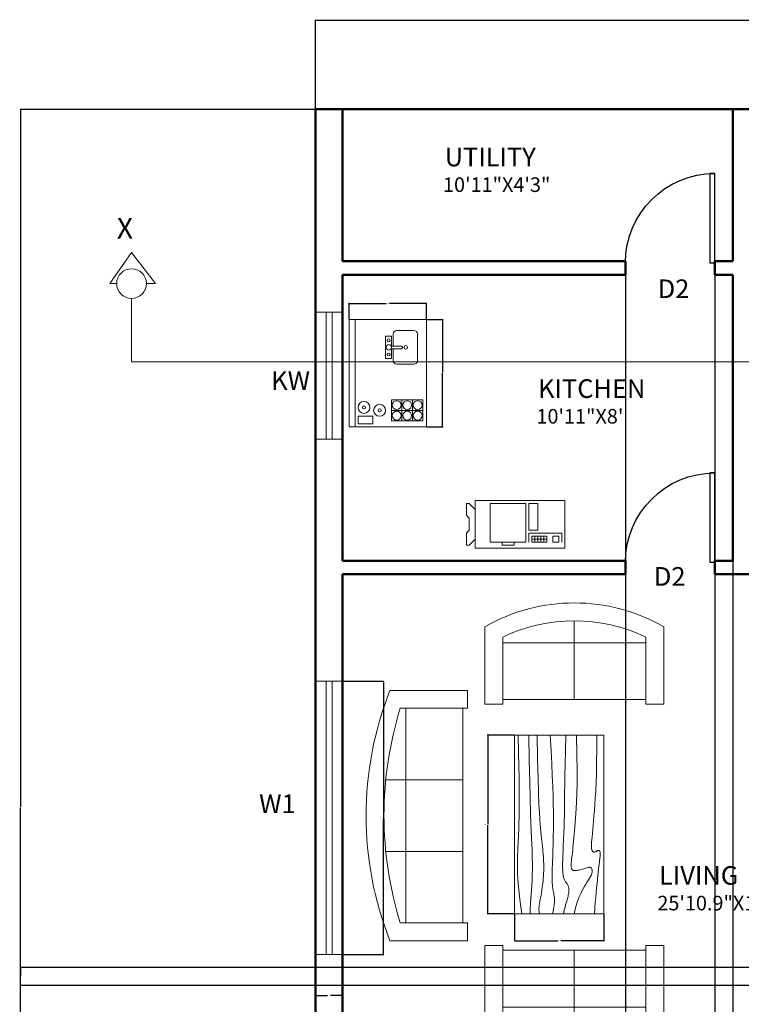
# Model space of a CAD drawing. Units: inches. Extents: x 7359 to 7979, y 33027 to 34263.
# Tile 31 of 32: x 7359 to 7601, y 33933 to 34263. Entities that reach past the tile are written whole.
import ezdxf

# ---------------------------------------------------------------- set-up
doc = ezdxf.new("R2010")
doc.units = ezdxf.units.IN
for name, color, linetype, lineweight in [('A-ANNO-DIMS', 2, 'Continuous', 18), ('A-ANNO-SYMB', 7, 'Continuous', 18), ('A-ANNO-TEXT', 3, 'Continuous', 18), ('A-AREA-IDEN', 7, 'Continuous', 18), ('A-DOOR', 3, 'Continuous', 25), ('A-EQPM', 8, 'Continuous', 18), ('A-FLOR-FIXT', 9, 'Continuous', 18), ('A-FURN', 8, 'Continuous', 18), ('A-GLAZ', 4, 'Continuous', 18), ('A-WALL', 7, 'Continuous', 50)]:
    doc.layers.add(name, color=color, linetype=linetype, lineweight=lineweight)
doc.styles.get("Standard").update_dxf_attribs({"font": 'arial.ttf'})
doc.dimstyles.get("Standard").update_dxf_attribs({"dimtxt": 0.18, "dimasz": 0.18, "dimexe": 0.18, "dimexo": 0.0625, "dimgap": 0.09, "dimtad": 0, "dimtih": 1, "dimtoh": 1, "dimdec": 4, "dimzin": 0, "dimdsep": 46, "dimtxsty": 'Standard', "dimcen": 0.09, "dimadec": 0, "dimazin": 0, "dimtfac": 1, "dimtdec": 4, "dimtofl": 0, "dimtmove": 0, "dimatfit": 3, "dimfxl": 1, "dimtolj": 1, "dimtzin": 0, "dimarcsym": 0})

# ---------------------------------------------------------------- blocks, each defined once
blk = doc.blocks.new('*U2')
for p, q in [((0, 0), (0, -100)), ((750, 0), (750, -100))]:
    blk.add_line(p, q)
blk.add_lwpolyline([(0, 0), (0, 750), (43.75, 750), (43.75, 0)], close=True)
blk.add_arc((0, 0), 750, 0, 90)
blk = doc.blocks.new('Table - Rectangular Woodgrain 60 x 30 in.')
for p, q in [((0, 0), (0, -30)), ((60, 0), (0, 0)), ((60, -30), (60, 0)), ((0, -30), (60, -30))]:
    blk.add_line(p, q)
for points in [[(0, -2.4), (4.8155, -2.418), (9.0302, -2.4688), (12.709, -2.5477), (15.9167, -2.65), (18.7181, -2.7711), (21.1781, -2.9063), (23.3616, -3.0508), (25.3333, -3.2), (27.1477, -3.3495), (28.8172, -3.4958), (30.3437, -3.636), (31.7291, -3.7667), (32.9756, -3.8849), (34.0849, -3.9875), (35.059, -4.0714), (35.9, -4.1334), (36.6114, -4.1711), (37.2041, -4.1854), (37.6906, -4.1779), (38.0833, -4.15), (38.3948, -4.1034), (38.6375, -4.0396), (38.8239, -3.9602), (38.9666, -3.8667), (39.0764, -3.7608), (39.1573, -3.6448), (39.2116, -3.521), (39.2416, -3.3917), (39.2498, -3.2593), (39.2385, -3.1261), (39.21, -2.9944), (39.1666, -2.8667), (39.111, -2.7447), (39.0468, -2.6281), (38.978, -2.5163), (38.9083, -2.4083), (38.8418, -2.3035), (38.7823, -2.201), (38.7337, -2.1001), (38.7, -2), (38.6844, -1.9003), (38.6875, -1.8021), (38.7094, -1.707), (38.75, -1.6167), (38.8094, -1.5326), (38.8875, -1.4563), (38.9844, -1.3893), (39.1, -1.3333), (39.2351, -1.2896), (39.3937, -1.2583), (39.5804, -1.2396), (39.8, -1.2333), (40.057, -1.2396), (40.3562, -1.2583), (40.7023, -1.2896), (41.1, -1.3333), (41.5547, -1.3895), (42.0755, -1.4573), (42.6721, -1.5361), (43.3542, -1.625), (44.1316, -1.7233), (45.014, -1.8302), (46.0114, -1.9449), (47.1333, -2.0667), (48.3862, -2.1947), (49.7625, -2.3281), (51.2513, -2.4663), (52.8416, -2.6083), (54.5226, -2.7535), (56.2833, -2.9011), (58.1127, -3.0501), (60, -3.2)], [(0, -9.2), (6.5759, -9.0858), (11.9385, -9.0365), (16.2527, -9.0418), (19.6833, -9.0917), (22.3952, -9.1759), (24.5531, -9.2844), (26.322, -9.4069), (27.8666, -9.5333), (29.3241, -9.6553), (30.7203, -9.7719), (32.0532, -9.8837), (33.3208, -9.9917), (34.5213, -10.0965), (35.6526, -10.199), (36.7128, -10.2999), (37.7, -10.4), (38.6129, -10.4996), (39.4531, -10.5969), (40.223, -10.6895), (40.925, -10.775), (41.5613, -10.8512), (42.1344, -10.9156), (42.6465, -10.966), (43.1, -11), (43.4976, -11.0158), (43.8437, -11.0136), (44.143, -10.9942), (44.4, -10.9583), (44.6195, -10.9069), (44.8062, -10.8406), (44.9648, -10.7603), (45.1, -10.6667), (45.2155, -10.5598), (45.3114, -10.4365), (45.3871, -10.2929), (45.4416, -10.125), (45.4743, -9.929), (45.4844, -9.7011), (45.4709, -9.4371), (45.4333, -9.1333), (45.3716, -8.7883), (45.2896, -8.4104), (45.1919, -8.0107), (45.0833, -7.6), (44.9685, -7.1893), (44.8521, -6.7896), (44.7388, -6.4117), (44.6333, -6.0667), (44.54, -5.7628), (44.4614, -5.4979), (44.4001, -5.2675), (44.3583, -5.0667), (44.3384, -4.8909), (44.3427, -4.7354), (44.3736, -4.5956), (44.4333, -4.4667), (44.5236, -4.3453), (44.6427, -4.2333), (44.7884, -4.1339), (44.9583, -4.05), (45.1501, -3.9849), (45.3614, -3.9417), (45.59, -3.9234), (45.8333, -3.9333), (46.0915, -3.9749), (46.3734, -4.0531), (46.6906, -4.1736), (47.0542, -4.3417), (47.4756, -4.5629), (47.9661, -4.8427), (48.5372, -5.1866), (49.2, -5.6), (49.9676, -6.0844), (50.8594, -6.625), (51.8965, -7.2031), (53.1, -7.8), (54.491, -8.3969), (56.0906, -8.975), (57.9199, -9.5156), (60, -10)], [(0, -12.8), (5.1847, -12.9322), (9.6213, -13.0323), (13.3963, -13.1059), (16.5958, -13.1583), (19.3063, -13.1952), (21.614, -13.2219), (23.6054, -13.2439), (25.3666, -13.2667), (26.9728, -13.2947), (28.4531, -13.3281), (29.8256, -13.3663), (31.1083, -13.4083), (32.3191, -13.4535), (33.476, -13.501), (34.597, -13.5501), (35.7, -13.6), (36.7984, -13.6497), (37.8875, -13.6979), (38.9578, -13.743), (40, -13.7833), (41.0047, -13.8174), (41.9625, -13.8438), (42.864, -13.8607), (43.7, -13.8667), (44.4631, -13.8604), (45.1552, -13.8417), (45.7801, -13.8104), (46.3416, -13.7667), (46.8439, -13.7104), (47.2906, -13.6417), (47.6858, -13.5604), (48.0333, -13.4667), (48.3375, -13.3608), (48.6042, -13.2448), (48.8396, -13.121), (49.05, -12.9917), (49.2417, -12.8593), (49.4208, -12.7261), (49.5937, -12.5944), (49.7667, -12.4667), (49.9452, -12.3451), (50.1323, -12.2313), (50.3303, -12.1268), (50.5416, -12.0333), (50.7686, -11.9524), (51.0135, -11.8854), (51.2788, -11.8341), (51.5666, -11.8), (51.8785, -11.7843), (52.2116, -11.7865), (52.562, -11.8059), (52.926, -11.8417), (53.2998, -11.8931), (53.6795, -11.9594), (54.0614, -12.0397), (54.4416, -12.1333), (54.8223, -12.2401), (55.2293, -12.3625), (55.6942, -12.5037), (56.2489, -12.6667), (56.9251, -12.8547), (57.7545, -13.0708), (58.7689, -13.3182), (60, -13.6)], [(0, -18), (5.124, -17.7273), (9.6609, -17.5057), (13.6705, -17.3303), (17.2125, -17.1958), (20.3467, -17.0973), (23.1328, -17.0297), (25.6307, -16.9878), (27.9, -16.9667), (29.9928, -16.9617), (31.9302, -16.9703), (33.7254, -16.9907), (35.3917, -17.0208), (36.9423, -17.0588), (38.3906, -17.1026), (39.7499, -17.1503), (41.0333, -17.2), (42.2519, -17.2496), (43.4073, -17.2969), (44.4986, -17.3395), (45.525, -17.375), (46.4858, -17.4012), (47.3802, -17.4156), (48.2074, -17.416), (48.9667, -17.4), (49.6583, -17.3662), (50.2872, -17.3167), (50.8595, -17.2547), (51.3812, -17.1833), (51.8584, -17.1057), (52.2971, -17.025), (52.7034, -16.9443), (53.0833, -16.8667), (53.443, -16.7951), (53.789, -16.7313), (54.128, -16.6768), (54.4666, -16.6334), (54.8115, -16.6024), (55.1693, -16.5854), (55.5465, -16.5841), (55.95, -16.6), (56.3828, -16.6337), (56.8346, -16.6823), (57.2915, -16.7418), (57.7396, -16.8084), (58.165, -16.878), (58.5539, -16.9469), (58.8924, -17.0111), (59.1666, -17.0667), (59.3679, -17.1107), (59.5078, -17.1438), (59.6032, -17.1675), (59.6708, -17.1833), (59.7275, -17.193), (59.7901, -17.1979), (59.8753, -17.1998), (60, -17.2)], [(0, -22.4), (8.0098, -22.2501), (14.4094, -22.1011), (19.4168, -21.9535), (23.25, -21.8083), (26.1269, -21.6663), (28.2656, -21.5281), (29.884, -21.3947), (31.2, -21.2667), (32.3967, -21.1448), (33.5172, -21.0292), (34.5697, -20.9198), (35.5625, -20.8167), (36.5037, -20.7198), (37.4015, -20.6292), (38.2642, -20.5448), (39.1, -20.4667), (39.9164, -20.3951), (40.7187, -20.3313), (41.5117, -20.2768), (42.3, -20.2333), (43.0883, -20.2024), (43.8812, -20.1854), (44.6836, -20.1841), (45.5, -20.2), (46.3328, -20.234), (47.1747, -20.2844), (48.0163, -20.3488), (48.8479, -20.425), (49.66, -20.5106), (50.4429, -20.6031), (51.1872, -20.7004), (51.8833, -20.8), (52.5246, -20.8999), (53.1166, -20.9995), (53.6681, -21.0983), (54.1875, -21.1958), (54.6834, -21.2919), (55.1646, -21.3859), (55.6394, -21.4777), (56.1167, -21.5667), (56.6028, -21.6515), (57.0961, -21.7266), (57.5929, -21.7852), (58.0896, -21.8208), (58.5823, -21.8268), (59.0674, -21.7964), (59.5412, -21.723), (60, -21.6)], [(0, -25.2), (8.6355, -25.0504), (15.7026, -24.9031), (21.4049, -24.7606), (25.9458, -24.625), (29.529, -24.4988), (32.3578, -24.3844), (34.6359, -24.284), (36.5667, -24.2), (38.3213, -24.1341), (39.9417, -24.0854), (41.437, -24.0523), (42.8167, -24.0333), (44.0901, -24.0268), (45.2667, -24.0313), (46.3557, -24.0451), (47.3667, -24.0667), (48.309, -24.0947), (49.1928, -24.1287), (50.0284, -24.168), (50.826, -24.2125), (51.5959, -24.2617), (52.3483, -24.3151), (53.0935, -24.3725), (53.8417, -24.4334), (54.6009, -24.497), (55.3699, -24.561), (56.1454, -24.6226), (56.9239, -24.6792), (57.7021, -24.7279), (58.4764, -24.7662), (59.2435, -24.7911), (60, -24.8)], [(0, -28.8), (5.6867, -28.6681), (10.45, -28.5698), (14.407, -28.5012), (17.675, -28.4584), (20.3711, -28.4374), (22.6125, -28.4344), (24.5164, -28.4455), (26.2, -28.4667), (27.762, -28.4947), (29.2276, -28.5281), (30.6033, -28.5663), (31.8958, -28.6084), (33.1118, -28.6535), (34.2578, -28.7011), (35.3405, -28.7501), (36.3666, -28.8), (37.3443, -28.8497), (38.288, -28.8974), (39.2137, -28.9412), (40.1375, -28.9792), (41.0753, -29.0093), (42.0432, -29.0297), (43.0572, -29.0384), (44.1333, -29.0333), (45.2936, -29.0114), (46.5843, -28.9641), (48.0579, -28.8816), (49.7666, -28.7542), (51.7629, -28.5721), (54.0989, -28.3255), (56.8272, -28.0048), (60, -27.6)]]:
    blk.add_lwpolyline(points)
blk = doc.blocks.new('Sofa - Roundback 7 ft.')
for p, q in [((-12.00002, -32.4421), (-12.00003, -6.5971)), ((11.99997, -32.4421), (11.99998, -6.5971)), ((-36.000027, -34), (-36.000027, -11.4696)), ((35.99998, -34), (35.99998, -11.4696)), ((-35.999844, -13.3819), (35.9998, -13.3819)), ((-36.000027, -32.4421), (35.99998, -32.4421))]:
    blk.add_line(p, q)
for points in [[(-36.000027, -34), (-42.000027, -34), (-42.000027, -8)], [(41.99998, -8), (41.99998, -34), (35.99998, -34)]]:
    blk.add_lwpolyline(points)
for centre, radius, start, end in [((0, -114.25), 114.25, 68.43141, 111.5686), ((-0.00001, -127.1968), 121.1968, 72.72033, 107.2797)]:
    blk.add_arc(centre, radius, start, end)
blk = doc.blocks.new('Sofa - Roundback Loveseat 5 ft.')
for p, q in [((0, -32.44198), (0, -5.99998)), ((-24, -33.99998), (-24, -11.46958)), ((24.00004, -33.99998), (24.00004, -11.46958)), ((-23.9998, -13.38178), (23.99986, -13.38178)), ((-24, -32.44198), (24.00004, -32.44198))]:
    blk.add_line(p, q)
for points in [[(-24, -33.99998), (-30, -33.99998), (-30, -7.99998)], [(30.00004, -7.99998), (30.00004, -33.99998), (24.00004, -33.99998)]]:
    blk.add_lwpolyline(points)
for centre, radius, start, end in [((0, -60.24998), 60.24998, 60.13715, 119.8628), ((0, -61.38438), 55.38444, 64.32083, 115.6792)]:
    blk.add_arc(centre, radius, start, end)
blk = doc.blocks.new('Wet Bar')
for p, q in [((0, 0), (36, 0)), ((0, -26), (0, 0)), ((36, 0), (36, -26)), ((0, -2), (36, -2)), ((3.5, -3), (1, -3)), ((1, -3), (1, -8)), ((3.5, -8), (3.5, -3)), ((1, -8), (3.5, -8)), ((2, -14.25), (9, -14.25)), ((2, -24.75), (2, -14.25)), ((5.5, -14.25), (5.5, -24.75)), ((9, -14.25), (9, -24.75)), ((26.2, -17.55), (26.2, -14.1284)), ((27.1001, -17.55), (27.1001, -14.1284)), ((2, -17.75), (9, -17.75)), ((9, -21.25), (2, -21.25)), ((36, -26), (0, -26)), ((9, -24.75), (2, -24.75))]:
    blk.add_line(p, q)
for points in [[(26.2, -14.25), (22.95, -14.25), (22.95, -12.2), (26.75, -12.2)], [(26.7487, -12.2), (30.3501, -12.2), (30.3501, -14.25), (27.1001, -14.25)], [(20.95, -21.75), (20.95, -16.05)], [(22.15, -14.85), (26.2, -14.85)], [(27.1001, -14.85), (31.15, -14.85)], [(32.3501, -16.05), (32.3501, -21.75)], [(31.15, -22.95), (22.15, -22.95)]]:
    blk.add_lwpolyline(points)
for centre, radius in [((6.5, -5), 2), ((6.5, -5), 0.5), ((5.5, -10.25), 2), ((5.5, -10.25), 0.5), ((24.25, -13.25), 0.5), ((26.65, -13.35), 0.9), ((29, -13.25), 0.5), ((3.75, -16), 1.5), ((7.25, -16), 1.5), ((3.75, -19.5), 1.5), ((7.25, -19.5), 1.5), ((26.65, -19.05), 0.6), ((3.75, -23), 1.5), ((7.25, -23), 1.5)]:
    blk.add_circle(centre, radius)
for centre, radius, start, end in [((22.2251, -16.125), 1.2772, 93.36646, 176.6335), ((31.075, -16.125), 1.2772, 3.366461, 86.63354), ((26.65, -17.55), 0.45, 180, 0), ((22.2251, -21.675), 1.2772, 183.3665, 266.6335), ((31.075, -21.675), 1.2772, 273.3665, 356.6335)]:
    blk.add_arc(centre, radius, start, end)
blk = doc.blocks.new('Copy Machine')
for p, q in [((0, 0), (0, -16)), ((30, 0), (0, 0)), ((30, -16), (30, 0)), ((-3, -1), (-3, -5)), ((-2, -1), (-3, -1)), ((0, -3), (-2, -1)), ((5, -1), (5, -14)), ((17, -1), (5, -1)), ((17, -14), (17, -1)), ((18, -1), (18, -10)), ((21, -1), (18, -1)), ((21, -10), (21, -1)), ((-3, -5), (-2, -6)), ((-2, -10), (-2, -6)), ((-3, -11), (-2, -10)), ((-3, -15), (-3, -11)), ((0, -13), (-2, -15)), ((18, -10), (21, -10)), ((18, -14), (18, -11)), ((18, -11), (29, -11)), ((24, -12), (19, -12)), ((19, -12), (19, -14)), ((24, -13), (19, -13)), ((20, -12), (20, -14)), ((21, -14), (21, -12)), ((22, -12), (22, -14)), ((23, -14), (23, -12)), ((24, -14), (24, -12)), ((28, -12), (26, -12)), ((26, -12), (26, -14)), ((28, -14), (28, -12)), ((29, -11), (29, -14)), ((-2, -15), (-3, -15)), ((0, -16), (30, -16)), ((5, -14), (17, -14)), ((9, -14), (9, -15)), ((9, -15), (13, -15)), ((13, -15), (13, -14)), ((19, -14), (24, -14)), ((26, -14), (28, -14))]:
    blk.add_line(p, q)
blk = doc.blocks.new('SECTION-HEAD')
for p, q in [((0, 4.98), (7.32, 15.43)), ((7.32, 15.43), (15.39, 4.98)), ((2.34, 4.98), (0, 4.98)), ((12.3, 4.98), (15.39, 4.98))]:
    blk.add_line(p, q)
blk.add_circle((7.32, 4.98), 4.98)
blk = doc.blocks.new('WINDOW-W1-LIVING')
for p, q in [((0, 91.75), (9, 91.75)), ((3.5, 0), (3.5, 91.75)), ((5.5, 0), (5.5, 91.75)), ((0, 0), (9, 0))]:
    blk.add_line(p, q)
blk = doc.blocks.new('WINDOW-KW')
for p, q in [((0, 42.66), (9, 42.66)), ((3.5, 42.66), (3.5, 0)), ((5.5, 42.66), (5.5, 0)), ((5.5, 42.66), (5.5, 0)), ((0, 0), (9, 0))]:
    blk.add_line(p, q)
blk = doc.blocks.new('*D38')
at = {"layer": 'A-ANNO-DIMS', "color": 0, "lineweight": -2, "transparency": 16777216}
for p, q in [((7525.29, 34023.33), (7516.18, 34023.33)), ((7516.36, 34023.15), (7516.36, 33993.51)), ((7516.36, 33963.51), (7516.36, 33993.14)), ((7525.29, 33963.33), (7516.18, 33963.33))]:
    blk.add_line(p, q, dxfattribs=at)
at = {"layer": 'A-ANNO-DIMS', "color": 0, "transparency": 16777216}
for points in [[(7516.33, 34023.15), (7516.39, 34023.15), (7516.36, 34023.33)], [(7516.33, 33963.51), (7516.39, 33963.51), (7516.36, 33963.33)]]:
    blk.add_solid(points, dxfattribs=at)
at = {"layer": 'Defpoints', "color": 0, "transparency": 16777216}
for p in [(7525.36, 34023.33), (7516.36, 33963.33), (7525.36, 33963.33)]:
    blk.add_point(p, dxfattribs=at)
at = {"layer": 'A-ANNO-DIMS', "color": 0, "transparency": 16777216, "insert": (7516.36, 33993.33), "char_height": 0.18, "attachment_point": 5}
blk.add_mtext('\\A1;COFFEE TABLE 60 TYP.', dxfattribs=at)
blk = doc.blocks.new('*D39')
at = {"layer": 'A-ANNO-DIMS', "color": 0, "lineweight": -2, "transparency": 16777216}
for p, q in [((7525.36, 33963.27), (7525.36, 33954.15)), ((7555.36, 33963.27), (7555.36, 33954.15)), ((7525.54, 33954.33), (7539.83, 33954.33)), ((7555.18, 33954.33), (7540.88, 33954.33))]:
    blk.add_line(p, q, dxfattribs=at)
at = {"layer": 'A-ANNO-DIMS', "color": 0, "transparency": 16777216}
for points in [[(7525.54, 33954.36), (7525.54, 33954.3), (7525.36, 33954.33)], [(7555.18, 33954.36), (7555.18, 33954.3), (7555.36, 33954.33)]]:
    blk.add_solid(points, dxfattribs=at)
at = {"layer": 'Defpoints', "color": 0, "transparency": 16777216}
for p in [(7525.36, 33963.33), (7555.36, 33963.33), (7555.36, 33954.33)]:
    blk.add_point(p, dxfattribs=at)
at = {"layer": 'A-ANNO-DIMS', "color": 0, "transparency": 16777216, "insert": (7540.36, 33954.33), "char_height": 0.18, "attachment_point": 5}
blk.add_mtext('\\A1;30 TYP.', dxfattribs=at)
blk = doc.blocks.new('*D42')
at = {"layer": 'A-ANNO-DIMS', "color": 0, "lineweight": -2, "transparency": 16777216}
for p, q in [((7495.88, 34162.81), (7501.4, 34162.81)), ((7501.22, 34162.63), (7501.22, 34144.99)), ((7501.22, 34126.99), (7501.22, 34144.63)), ((7495.88, 34126.81), (7501.4, 34126.81))]:
    blk.add_line(p, q, dxfattribs=at)
at = {"layer": 'A-ANNO-DIMS', "color": 0, "transparency": 16777216}
for points in [[(7501.19, 34162.63), (7501.25, 34162.63), (7501.22, 34162.81)], [(7501.19, 34126.99), (7501.25, 34126.99), (7501.22, 34126.81)]]:
    blk.add_solid(points, dxfattribs=at)
at = {"layer": 'Defpoints', "color": 0, "transparency": 16777216}
for p in [(7495.82, 34162.81), (7501.22, 34162.81), (7495.82, 34126.81)]:
    blk.add_point(p, dxfattribs=at)
at = {"layer": 'A-ANNO-DIMS', "color": 0, "transparency": 16777216, "insert": (7501.22, 34144.81), "char_height": 0.18, "attachment_point": 5}
blk.add_mtext('\\A1;WET BAR 36 TYP.', dxfattribs=at)
blk = doc.blocks.new('*D43')
at = {"layer": 'A-ANNO-DIMS', "color": 0, "lineweight": -2, "transparency": 16777216}
for p, q in [((7469.82, 34162.87), (7469.82, 34168.39)), ((7470, 34168.21), (7482.29, 34168.21)), ((7495.64, 34168.21), (7483.35, 34168.21)), ((7495.82, 34162.87), (7495.82, 34168.39))]:
    blk.add_line(p, q, dxfattribs=at)
at = {"layer": 'A-ANNO-DIMS', "color": 0, "transparency": 16777216}
for points in [[(7470, 34168.24), (7470, 34168.18), (7469.82, 34168.21)], [(7495.64, 34168.24), (7495.64, 34168.18), (7495.82, 34168.21)]]:
    blk.add_solid(points, dxfattribs=at)
at = {"layer": 'Defpoints', "color": 0, "transparency": 16777216}
for p in [(7469.82, 34168.21), (7469.82, 34162.81), (7495.82, 34162.81)]:
    blk.add_point(p, dxfattribs=at)
at = {"layer": 'A-ANNO-DIMS', "color": 0, "transparency": 16777216, "insert": (7482.82, 34168.21), "char_height": 0.18, "attachment_point": 5}
blk.add_mtext('\\A1;26 TYP.', dxfattribs=at)
blk = doc.blocks.new('*D56')
at = {"layer": 'A-ANNO-DIMS', "color": 0, "lineweight": -2, "transparency": 16777216}
for p, q in [((7467.65, 34041.43), (7481.53, 34041.43)), ((7481.35, 34041.25), (7481.35, 33995.74)), ((7481.35, 33949.87), (7481.35, 33995.38)), ((7467.65, 33949.69), (7481.53, 33949.69))]:
    blk.add_line(p, q, dxfattribs=at)
at = {"layer": 'A-ANNO-DIMS', "color": 0, "transparency": 16777216}
for points in [[(7481.32, 34041.25), (7481.38, 34041.25), (7481.35, 34041.43)], [(7481.32, 33949.87), (7481.38, 33949.87), (7481.35, 33949.69)]]:
    blk.add_solid(points, dxfattribs=at)
at = {"layer": 'Defpoints', "color": 0, "transparency": 16777216}
for p in [(7467.59, 34041.43), (7481.35, 34041.43), (7467.59, 33949.69)]:
    blk.add_point(p, dxfattribs=at)
at = {"layer": 'A-ANNO-DIMS', "color": 0, "transparency": 16777216, "insert": (7481.35, 33995.56), "char_height": 0.18, "attachment_point": 5}
blk.add_mtext('\\A1;LIVING W1 92 TYP.', dxfattribs=at)
blk = doc.blocks.new('*D57')
at = {"layer": 'A-ANNO-DIMS', "color": 0, "lineweight": -2, "transparency": 16777216}
for p, q in [((7458.59, 33949.62), (7458.59, 33935.75)), ((7467.59, 33949.62), (7467.59, 33935.75)), ((7458.77, 33935.93), (7462.63, 33935.93)), ((7467.41, 33935.93), (7463.55, 33935.93))]:
    blk.add_line(p, q, dxfattribs=at)
at = {"layer": 'A-ANNO-DIMS', "color": 0, "transparency": 16777216}
for points in [[(7458.77, 33935.96), (7458.77, 33935.9), (7458.59, 33935.93)], [(7467.41, 33935.96), (7467.41, 33935.9), (7467.59, 33935.93)]]:
    blk.add_solid(points, dxfattribs=at)
at = {"layer": 'Defpoints', "color": 0, "transparency": 16777216}
for p in [(7458.59, 33949.69), (7467.59, 33949.69), (7467.59, 33935.93)]:
    blk.add_point(p, dxfattribs=at)
at = {"layer": 'A-ANNO-DIMS', "color": 0, "transparency": 16777216, "insert": (7463.09, 33935.93), "char_height": 0.18, "attachment_point": 5}
blk.add_mtext('\\A1;9 TYP.', dxfattribs=at)
blk = doc.blocks.new('*D64')
at = {"layer": 'A-ANNO-DIMS', "color": 0, "lineweight": -2, "transparency": 16777216}
for p, q in [((7458.59, 34233.4), (7458.59, 34263.41)), ((7458.77, 34263.23), (7670.89, 34263.23)), ((7883.81, 34263.23), (7671.69, 34263.23)), ((7883.99, 34233.4), (7883.99, 34263.41))]:
    blk.add_line(p, q, dxfattribs=at)
at = {"layer": 'A-ANNO-DIMS', "color": 0, "transparency": 16777216}
for points in [[(7458.77, 34263.26), (7458.77, 34263.2), (7458.59, 34263.23)], [(7883.81, 34263.26), (7883.81, 34263.2), (7883.99, 34263.23)]]:
    blk.add_solid(points, dxfattribs=at)
at = {"layer": 'Defpoints', "color": 0, "transparency": 16777216}
for p in [(7883.99, 34263.23), (7458.59, 34233.33), (7883.99, 34233.33)]:
    blk.add_point(p, dxfattribs=at)
at = {"layer": 'A-ANNO-DIMS', "color": 0, "transparency": 16777216, "insert": (7671.29, 34263.23), "char_height": 0.18, "attachment_point": 5}
blk.add_mtext('\\A1;425.4', dxfattribs=at)
blk = doc.blocks.new('*D65')
at = {"layer": 'A-ANNO-DIMS', "color": 0, "lineweight": -2, "transparency": 16777216}
for p, q in [((7458.53, 34233.33), (7359.41, 34233.33)), ((7359.59, 34233.15), (7359.59, 33999.27)), ((7359.59, 33765.01), (7359.59, 33998.9)), ((7458.53, 33764.83), (7359.41, 33764.83))]:
    blk.add_line(p, q, dxfattribs=at)
at = {"layer": 'A-ANNO-DIMS', "color": 0, "transparency": 16777216}
for points in [[(7359.56, 34233.15), (7359.62, 34233.15), (7359.59, 34233.33)], [(7359.56, 33765.01), (7359.62, 33765.01), (7359.59, 33764.83)]]:
    blk.add_solid(points, dxfattribs=at)
at = {"layer": 'Defpoints', "color": 0, "transparency": 16777216}
for p in [(7359.59, 34233.33), (7458.59, 34233.33), (7458.59, 33764.83)]:
    blk.add_point(p, dxfattribs=at)
at = {"layer": 'A-ANNO-DIMS', "color": 0, "transparency": 16777216, "insert": (7359.59, 33999.08), "char_height": 0.18, "attachment_point": 5}
blk.add_mtext('\\A1;468.5', dxfattribs=at)
blk = doc.blocks.new('*D68')
at = {"layer": 'A-ANNO-DIMS', "color": 0, "lineweight": -2, "transparency": 16777216}
for p, q in [((7562.59, 34181.77), (7562.59, 33632.31)), ((7592.59, 34181.77), (7592.59, 33632.31)), ((7562.77, 33632.49), (7577.37, 33632.49)), ((7592.41, 33632.49), (7577.81, 33632.49))]:
    blk.add_line(p, q, dxfattribs=at)
at = {"layer": 'A-ANNO-DIMS', "color": 0, "transparency": 16777216}
for points in [[(7562.77, 33632.52), (7562.77, 33632.46), (7562.59, 33632.49)], [(7592.41, 33632.52), (7592.41, 33632.46), (7592.59, 33632.49)]]:
    blk.add_solid(points, dxfattribs=at)
at = {"layer": 'Defpoints', "color": 0, "transparency": 16777216}
for p in [(7562.59, 34181.83), (7592.59, 34181.83), (7592.59, 33632.49)]:
    blk.add_point(p, dxfattribs=at)
at = {"layer": 'A-ANNO-DIMS', "color": 0, "transparency": 16777216, "insert": (7577.59, 33632.49), "char_height": 0.18, "attachment_point": 5}
blk.add_mtext('\\A1;30', dxfattribs=at)
blk = doc.blocks.new('*D83')
at = {"layer": 'A-ANNO-DIMS', "color": 0, "lineweight": -2, "transparency": 16777216}
for p, q in [((7592.591484, 34081.771428), (7592.591484, 33632.309146)), ((7598.591484, 34081.771428), (7598.591484, 33632.309146)), ((7592.771484, 33632.489146), (7595.442057, 33632.489146)), ((7598.411484, 33632.489146), (7595.740911, 33632.489146))]:
    blk.add_line(p, q, dxfattribs=at)
at = {"layer": 'A-ANNO-DIMS', "color": 0, "transparency": 16777216}
for points in [[(7592.771484, 33632.519146), (7592.771484, 33632.459146), (7592.591484, 33632.489146)], [(7598.411484, 33632.519146), (7598.411484, 33632.459146), (7598.591484, 33632.489146)]]:
    blk.add_solid(points, dxfattribs=at)
at = {"layer": 'Defpoints', "color": 0, "transparency": 16777216}
for p in [(7592.591484, 34081.833928), (7598.591484, 34081.833928), (7598.591484, 33632.489146)]:
    blk.add_point(p, dxfattribs=at)
at = {"layer": 'A-ANNO-DIMS', "color": 0, "transparency": 16777216, "insert": (7595.591484, 33632.489146), "char_height": 0.18, "attachment_point": 5}
blk.add_mtext('\\A1;6', dxfattribs=at)
blk = doc.blocks.new('*D84')
at = {"layer": 'A-ANNO-DIMS', "color": 0, "lineweight": -2, "transparency": 16777216}
for p, q in [((7782.93, 33945.33), (7359.41, 33945.33)), ((7359.59, 33945.15), (7359.59, 33942.52)), ((7359.59, 33939.51), (7359.59, 33942.15)), ((7782.93, 33939.33), (7359.41, 33939.33))]:
    blk.add_line(p, q, dxfattribs=at)
at = {"layer": 'A-ANNO-DIMS', "color": 0, "transparency": 16777216}
for points in [[(7359.56, 33945.15), (7359.62, 33945.15), (7359.59, 33945.33)], [(7359.56, 33939.51), (7359.62, 33939.51), (7359.59, 33939.33)]]:
    blk.add_solid(points, dxfattribs=at)
at = {"layer": 'Defpoints', "color": 0, "transparency": 16777216}
for p in [(7782.99, 33945.33), (7359.59, 33939.33), (7782.99, 33939.33)]:
    blk.add_point(p, dxfattribs=at)
at = {"layer": 'A-ANNO-DIMS', "color": 0, "transparency": 16777216, "insert": (7359.59, 33942.33), "char_height": 0.18, "attachment_point": 5}
blk.add_mtext('\\A1;6', dxfattribs=at)

msp = doc.modelspace()

# ---------------------------------------------------------------- linework, layer by layer
at = {"layer": 'A-ANNO-SYMB'}
for q in [(7396.8072, 34169.8623), (7930.5345, 34148.6536)]:
    msp.add_line((7396.8072, 34148.6536), q, dxfattribs=at)
at = {"layer": 'A-WALL'}
for p, q in [((7458.5915, 34233.3339), (7883.9915, 34233.3339)), ((7458.5915, 34233.3339), (7458.5915, 33764.8339)), ((7467.5915, 34233.3339), (7467.5915, 34182.3339)), ((7598.5915, 34233.3339), (7598.5915, 34182.3339)), ((7467.5915, 34182.3339), (7562.5915, 34182.3339)), ((7562.5915, 34182.3339), (7562.5915, 34177.8339)), ((7592.5915, 34182.3339), (7592.5915, 34177.8339)), ((7592.5915, 34182.3339), (7598.5915, 34182.3339)), ((7467.5915, 34177.8339), (7562.5915, 34177.8339)), ((7467.5915, 34177.8339), (7467.5915, 34081.8339)), ((7592.5915, 34177.8339), (7598.5915, 34177.8339)), ((7598.5915, 34177.8339), (7598.5915, 34081.8339)), ((7467.5915, 34081.8339), (7562.5915, 34081.8339)), ((7562.5915, 34081.8339), (7562.5915, 34077.3339)), ((7592.5915, 34081.8339), (7592.5915, 34077.3339)), ((7592.5915, 34081.8339), (7598.5915, 34081.8339)), ((7467.5915, 34077.3339), (7562.5915, 34077.3339)), ((7467.5915, 34077.3339), (7467.5915, 33907.2339)), ((7592.5915, 34077.3339), (7681.0915, 34077.3339))]:
    msp.add_line(p, q, dxfattribs=at)

# ---------------------------------------------------------------- block references
at = {"layer": 'A-ANNO-SYMB'}
msp.add_blockref('SECTION-HEAD', (7389.487, 34169.862), dxfattribs=at)
at = {"layer": 'A-DOOR', "xscale": -0.0399999999999999, "yscale": 0.0399999999999999, "zscale": 0.0399999999999999}
for p in [(7592.5915, 34181.8339), (7592.5915, 34081.3339)]:
    msp.add_blockref('*U2', p, dxfattribs=at)
at = {"layer": 'A-EQPM'}
msp.add_blockref('Copy Machine', (7512.1732, 34102.092), dxfattribs=at)
at = {"layer": 'A-FLOR-FIXT', "rotation": 90}
msp.add_blockref('Wet Bar', (7469.8188, 34126.8098), dxfattribs=at)
at = {"layer": 'A-FURN'}
msp.add_blockref('Sofa - Roundback Loveseat 5 ft.', (7545.3969, 34067.6916), dxfattribs=at)
for name, p, rotation in [('Sofa - Roundback 7 ft.', (7475.537, 33996.3257), 90), ('Table - Rectangular Woodgrain 60 x 30 in.', (7555.3569, 34023.328), 270)]:
    msp.add_blockref(name, p, dxfattribs=dict(at, rotation=rotation))
at = {"layer": 'A-FURN', "xscale": -1, "rotation": 180}
msp.add_blockref('Sofa - Roundback Loveseat 5 ft.', (7545.3969, 33918.6792), dxfattribs=at)
at = {"layer": 'A-GLAZ'}
for name, p in [('WINDOW-KW', (7458.591, 34122.656)), ('WINDOW-W1-LIVING', (7458.591, 33949.687))]:
    msp.add_blockref(name, p, dxfattribs=at)

# ---------------------------------------------------------------- texts
at = {"layer": 'A-ANNO-SYMB'}
msp.add_text('X', height=6.9459, dxfattribs=at).set_placement((7391.8869, 34189.9559))
at = {"layer": 'A-ANNO-TEXT'}
for s, p in [('D2', (7573.4016, 34169.9806)), ('KW', (7443.6959, 34139.19)), ('D2', (7572.1218, 34073.4521)), ('W1', (7439.6456, 33997.1438))]:
    msp.add_text(s, height=6.25941, dxfattribs=at).set_placement(p)
at = {"layer": 'A-AREA-IDEN'}
for s, height, p in [('UTILITY', 6.25941, (7501.9082, 34214.2019)), ('10\'11"X4\'3"', 4.885549, (7501.3449, 34205.6075)), ('KITCHEN', 6.25941, (7533.2597, 34136.4807)), ('10\'11"X8\'', 4.88555, (7532.6964, 34127.8863)), ('LIVING', 6.25941, (7573.8371, 33973.1071)), ('25\'10.9"X14\'1.6"', 4.885549, (7573.2739, 33964.5127))]:
    msp.add_text(s, height=height, dxfattribs=at).set_placement(p)

# ---------------------------------------------------------------- dimensions: what is measured, and where the dimension line sits
at = {"layer": 'A-ANNO-DIMS'}
for base, p1, p2, override, picture, middle in [((7883.9915, 34263.2339), (7458.5915, 34233.3339), (7883.9915, 34233.3339), {"dimdec": 1, "dimlfac": 1, "dimrnd": 0, "dimzin": 0, "dimdsep": 46, "dimlunit": 2}, '*D64', (7671.2915, 34263.2339)), ((7592.5915, 33632.4891), (7562.5915, 34181.8339), (7592.5915, 34181.8339), {"dimdec": 0, "dimlfac": 1, "dimrnd": 0, "dimzin": 0, "dimdsep": 46, "dimlunit": 2}, '*D68', (7577.5915, 33632.4891)), ((7598.5915, 33632.4891), (7592.5915, 34081.8339), (7598.5915, 34081.8339), {"dimdec": 0, "dimlfac": 1, "dimrnd": 0, "dimzin": 0, "dimdsep": 46, "dimlunit": 2}, '*D83', (7595.5915, 33632.4891))]:
    dim = msp.add_linear_dim(base=base, p1=p1, p2=p2, dimstyle='Standard', override=override, dxfattribs=at)
    dim.commit()
    dim.dimension.update_dxf_attribs({"geometry": picture, "text_midpoint": middle})
for base, p1, p2, override, picture, middle in [((7359.5866, 34233.3339), (7458.5915, 33764.8339), (7458.5915, 34233.3339), {"dimdec": 1, "dimlfac": 1, "dimrnd": 0, "dimzin": 0, "dimdsep": 46, "dimlunit": 2}, '*D65', (7359.5866, 33999.0839)), ((7359.5866, 33939.3339), (7782.9915, 33945.3339), (7782.9915, 33939.3339), {"dimdec": 0, "dimlfac": 1, "dimrnd": 0, "dimzin": 0, "dimdsep": 46, "dimlunit": 2}, '*D84', (7359.5866, 33942.3339))]:
    dim = msp.add_linear_dim(base=base, p1=p1, p2=p2, angle=90, dimstyle='Standard', override=override, dxfattribs=at)
    dim.commit()
    dim.dimension.update_dxf_attribs({"geometry": picture, "text_midpoint": middle})
for base, p1, p2, angle, text, picture, middle in [((7469.8188, 34168.2098), (7495.8188, 34162.8098), (7469.8188, 34162.8098), 180, '<> TYP.', '*D43', (7482.8188, 34168.2098)), ((7501.2188, 34162.8098), (7495.8188, 34126.8098), (7495.8188, 34162.8098), 90, 'WET BAR <> TYP.', '*D42', (7501.2188, 34144.8098)), ((7481.3533, 34041.4329), (7467.5915, 33949.6873), (7467.5915, 34041.4329), 90, 'LIVING W1 <> TYP.', '*D56', (7481.3533, 33995.5601)), ((7516.3569, 33963.328), (7525.3569, 34023.328), (7525.3569, 33963.328), 270, 'COFFEE TABLE <> TYP.', '*D38', (7516.3569, 33993.328))]:
    dim = msp.add_linear_dim(base=base, p1=p1, p2=p2, angle=angle, text=text, dimstyle='Standard', override={"dimdec": 0, "dimlfac": 1, "dimrnd": 0, "dimzin": 0, "dimdsep": 46, "dimlunit": 2}, dxfattribs=at)
    dim.commit()
    dim.dimension.update_dxf_attribs({"geometry": picture, "text_midpoint": middle})
for base, p1, p2, picture, middle in [((7555.3569, 33954.328), (7525.3569, 33963.328), (7555.3569, 33963.328), '*D39', (7540.3569, 33954.328)), ((7467.5915, 33935.9255), (7458.5915, 33949.6873), (7467.5915, 33949.6873), '*D57', (7463.0915, 33935.9255))]:
    dim = msp.add_linear_dim(base=base, p1=p1, p2=p2, text='<> TYP.', dimstyle='Standard', override={"dimdec": 0, "dimlfac": 1, "dimrnd": 0, "dimzin": 0, "dimdsep": 46, "dimlunit": 2}, dxfattribs=at)
    dim.commit()
    dim.dimension.update_dxf_attribs({"geometry": picture, "text_midpoint": middle})

doc.saveas('drawing.dxf')
